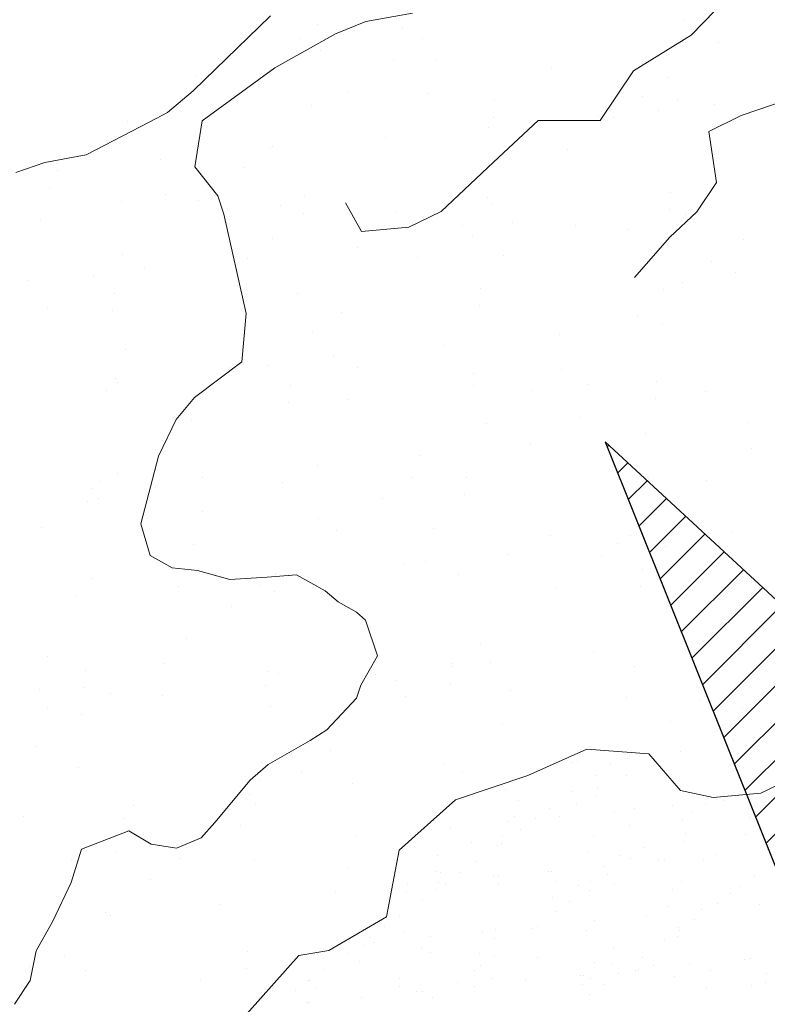
# Model space of a CAD drawing. Units: inches. Extents: x 1986 to 21484, y -1816 to 2016.
# Tile 62 of 85: x 3651.423 to 3655.81, y 1892.891 to 1898.672. Entities that reach past the tile are written whole.
import ezdxf

# ---------------------------------------------------------------- set-up
doc = ezdxf.new("R2010")
doc.units = ezdxf.units.IN
doc.layers.add('L-PLNT', color=84, linetype='Continuous', lineweight=13)
doc.layers.add('vfolhas', color=114, linetype='Continuous', lineweight=5)
doc.layers.add('vfolhas2', color=102, linetype='Continuous')

# ---------------------------------------------------------------- blocks, each defined once
blk = doc.blocks.new('arbusto_PB_verde_grande')
at = {"layer": 'vfolhas'}
h = blk.add_hatch(dxfattribs=at)
h.set_pattern_fill('ANSI31', color=256, scale=0.05, style=0)
h.set_pattern_definition([(45, (-2446.5133113, 50.986076), (-0.004419417382, 0.004419417382), [])])
h.paths.add_polyline_path([(-0.07279, 0.50669), (-0.18085, 0.65063), (-0.2334, 0.67253), (-0.20712, 0.53176), (-0.10785, 0.25007), (0.02625, -0.03934), (0.00028, 0.09048), (0.00816, 0.16241), (-0.04939, 0.29079)])
h.paths.add_polyline_path([(0.09902, 0.41929), (0.09372, 0.26573), (0.07906, 0.18814), (0.15506, 0.36901), (0.26606, 0.5505), (0.28356, 0.63504), (0.2485, 0.68819), (0.25145, 0.63504), (0.20178, 0.54426)])
h.paths.add_polyline_path([(0.12295, 0.24073), (0.047, 0.06233), (0.02625, -0.03934), (0.11122, 0.04358), (0.18428, 0.09364), (0.27478, 0.19376), (0.3215, 0.25323), (0.44129, 0.38467), (0.47634, 0.57866), (0.41789, 0.45347), (0.28939, 0.30954)])
h.paths.add_polyline_path([(0.58145, -0.03779), (0.70707, 0.01536), (0.78591, 0.04667), (0.74796, 0.06549), (0.62818, 0.08423), (0.52595, 0.09048), (0.39745, 0.04358), (0.02625, -0.03934), (0.25728, -0.03154), (0.43834, -0.0347)])
h.paths.add_polyline_path([(0.52022, -0.03647), (0.43834, -0.0347), (0.25728, -0.03154), (0.02625, -0.03934), (0.17964, -0.08515), (0.53768, -0.13167), (0.69541, -0.15357), (0.78591, -0.07852), (0.70413, -0.10042)])
h.paths.add_polyline_path([(0.27189, -0.21929), (0.14922, -0.14107), (0.02625, -0.03934), (0.15794, -0.31007), (0.29522, -0.42585), (0.41789, -0.49157), (0.56396, -0.56669), (0.5114, -0.48532), (0.39456, -0.34139)])
h.paths.add_polyline_path([(-0.05818, -0.47591), (-0.02312, -0.61984), (0.047, -0.80134), (0.08494, -0.59794), (0.07911, -0.4071), (0.03527, -0.25376), (0.02625, -0.03934), (-0.03773, -0.26001)])
h.paths.add_polyline_path([(-0.24218, 0.14054), (-0.11073, 0.06858), (0.02625, -0.03934), (-0.04235, 0.10871), (-0.21007, 0.23757), (-0.36485, 0.33145), (-0.47874, 0.40341), (-0.54303, 0.46288), (-0.49041, 0.33145), (-0.39408, 0.22192)])
at = {"layer": 'vfolhas2'}
for p, q in [((-0.54303, 0.46288), (-0.49041, 0.33145)), ((-0.47874, 0.40341), (-0.54303, 0.46288))]:
    blk.add_line(p, q, dxfattribs=at)
blk = doc.blocks.new('PLANT-SHRUB')
for p, q in [((2167.3863, 1874.3284), (2167.3863, 1874.3284)), ((2167.3494, 1874.2947), (2167.3494, 1874.2947)), ((2167.4592, 1874.2897), (2167.4592, 1874.2897)), ((2167.3538, 1874.1683), (2167.3538, 1874.1683)), ((2167.3823, 1874.1464), (2167.3823, 1874.1464)), ((2167.6597, 1874.1135), (2167.6597, 1874.1135)), ((2167.5754, 1874.0598), (2167.5754, 1874.0598)), ((2167.1002, 1873.9682), (2167.1002, 1873.9682)), ((2167.64, 1873.9488), (2167.64, 1873.9488)), ((2167.7513, 1873.937), (2167.7513, 1873.937)), ((2167.0085, 1873.8316), (2167.0085, 1873.8316)), ((2167.1125, 1873.8179), (2167.1125, 1873.8179)), ((2167.1125, 1873.8179), (2167.1125, 1873.8179)), ((2167.1794, 1873.8075), (2167.1794, 1873.8075)), ((2167.8017, 1873.8064), (2167.8017, 1873.8064)), ((2166.8467, 1873.7681), (2166.8467, 1873.7681)), ((2166.8467, 1873.7681), (2166.8467, 1873.7681)), ((2167.2749, 1873.7965), (2167.2749, 1873.7965)), ((2167.3697, 1873.7614), (2167.3697, 1873.7614)), ((2167.4374, 1873.7751), (2167.4374, 1873.7751)), ((2167.5464, 1873.7608), (2167.5464, 1873.7608)), ((2167.5774, 1873.7777), (2167.5774, 1873.7777)), ((2167.6504, 1873.7471), (2167.6504, 1873.7471)), ((2167.8809, 1873.7638), (2167.8809, 1873.7638)), ((2167.8928, 1873.7547), (2167.8928, 1873.7547)), ((2167.5406, 1873.744), (2167.5406, 1873.744)), ((2167.8129, 1873.7257), (2167.8129, 1873.7257)), ((2167.9803, 1873.7037), (2167.9803, 1873.7037)), ((2168.0843, 1873.69), (2168.0843, 1873.69)), ((2167.9692, 1873.6361), (2167.9692, 1873.6361)), ((2168.1883, 1873.6763), (2168.1883, 1873.6763)), ((2168.1883, 1873.6763), (2168.1883, 1873.6763)), ((2166.876, 1873.6143), (2166.876, 1873.6143)), ((2167.0876, 1873.5831), (2167.0876, 1873.5831)), ((2167.4983, 1873.6131), (2167.4983, 1873.6131)), ((2168.1206, 1873.612), (2168.1206, 1873.612)), ((2168.1782, 1873.6023), (2168.1782, 1873.6023)), ((2166.4493, 1873.5617), (2166.6467, 1873.5)), ((2166.7917, 1873.5606), (2166.7917, 1873.5606)), ((2167.1598, 1873.5541), (2167.1598, 1873.5541)), ((2167.3417, 1873.5617), (2167.3417, 1873.5617)), ((2167.414, 1873.5594), (2167.414, 1873.5594)), ((2167.6274, 1873.5637), (2167.6274, 1873.5637)), ((2167.8955, 1873.5686), (2167.8955, 1873.5686)), ((2168.0363, 1873.5583), (2168.0363, 1873.5583)), ((2168.1413, 1873.5686), (2168.1413, 1873.5686)), ((2168.1505, 1873.557), (2168.1505, 1873.557)), ((2166.6467, 1873.5), (2166.8689, 1873.3274)), ((2167.1678, 1873.4024), (2167.1678, 1873.4024)), ((2166.8341, 1873.383), (2166.8341, 1873.383)), ((2167.131, 1873.3687), (2167.131, 1873.3687)), ((2167.3286, 1873.3982), (2167.3286, 1873.3982)), ((2167.3572, 1873.3763), (2167.3572, 1873.3763)), ((2167.8684, 1873.3788), (2167.8684, 1873.3788)), ((2167.9424, 1873.3863), (2167.9424, 1873.3863)), ((2168.4081, 1873.3593), (2168.4081, 1873.3593)), ((2168.4081, 1873.3593), (2168.4081, 1873.3593)), ((2166.8689, 1873.3274), (2166.9799, 1873.1671)), ((2166.9282, 1873.3248), (2166.9282, 1873.3248)), ((2167.018, 1873.3071), (2167.018, 1873.3071)), ((2167.0907, 1873.3034), (2167.0907, 1873.3034)), ((2167.6403, 1873.306), (2167.6403, 1873.306)), ((2168.2626, 1873.3049), (2168.2626, 1873.3049)), ((2167.3621, 1873.2676), (2167.3621, 1873.2676)), ((2167.4661, 1873.254), (2167.4661, 1873.254)), ((2167.6286, 1873.2326), (2167.6286, 1873.2326)), ((2167.7686, 1873.227), (2167.7686, 1873.227)), ((2167.0751, 1873.1981), (2167.0751, 1873.1981)), ((2167.4977, 1873.2041), (2167.4977, 1873.2041)), ((2167.6148, 1873.1787), (2167.6148, 1873.1787)), ((2167.7317, 1873.1933), (2167.7317, 1873.1933)), ((2167.9, 1873.1968), (2167.9, 1873.1968)), ((2168.0041, 1873.1831), (2168.0041, 1873.1831)), ((2168.1379, 1873.172), (2168.1379, 1873.172)), ((2168.5431, 1873.2109), (2168.5431, 1873.2109)), ((2168.6491, 1873.1744), (2168.6491, 1873.1744)), ((2166.5531, 1873.1675), (2166.5531, 1873.1675)), ((2166.9799, 1873.1671), (2166.9676, 1872.8834)), ((2167.3369, 1873.1127), (2167.3369, 1873.1127)), ((2167.7977, 1873.1653), (2167.7977, 1873.1653)), ((2167.9592, 1873.1116), (2167.9592, 1873.1116)), ((2168.1665, 1873.1617), (2168.1665, 1873.1617)), ((2168.438, 1873.126), (2168.438, 1873.126)), ((2168.542, 1873.1123), (2168.542, 1873.1123)), ((2168.5815, 1873.1105), (2168.5815, 1873.1105)), ((2166.3845, 1873.0602), (2166.3845, 1873.0602)), ((2167.2526, 1873.059), (2167.2526, 1873.059)), ((2167.6292, 1873.0579), (2167.6292, 1873.0579)), ((2167.875, 1873.0579), (2167.875, 1873.0579)), ((2168.4973, 1873.0568), (2168.4973, 1873.0568)), ((2168.7044, 1873.0909), (2168.7044, 1873.0909)), ((2168.8738, 1873.0556), (2168.8738, 1873.0556)), ((2166.8215, 1872.998), (2166.8215, 1872.998)), ((2167.5328, 1873.011), (2167.5328, 1873.011)), ((2168.3325, 1873.0179), (2168.3325, 1873.0179)), ((2168.3693, 1873.0516), (2168.3693, 1873.0516)), ((2167.3446, 1872.9913), (2167.3446, 1872.9913)), ((2167.8558, 1872.9937), (2167.8558, 1872.9937)), ((2167.8677, 1872.9846), (2167.8677, 1872.9846)), ((2168.3955, 1872.9743), (2168.3955, 1872.9743)), ((2168.8901, 1872.9895), (2168.8901, 1872.9895)), ((2168.9186, 1872.9676), (2168.9186, 1872.9676)), ((2166.9676, 1872.8834), (2167.2144, 1872.6121)), ((2167.15, 1872.8855), (2167.15, 1872.8855)), ((2166.536, 1872.859), (2166.536, 1872.859)), ((2166.744, 1872.8316), (2166.744, 1872.8316)), ((2167.359, 1872.8517), (2167.359, 1872.8517)), ((2168.1336, 1872.8356), (2168.1336, 1872.8356)), ((2168.6992, 1872.8533), (2168.6992, 1872.8533)), ((2168.9332, 1872.8425), (2168.9332, 1872.8425)), ((2168.97, 1872.8762), (2168.97, 1872.8762)), ((2167.0625, 1872.8131), (2167.0625, 1872.8131)), ((2167.0689, 1872.7888), (2167.0689, 1872.7888)), ((2167.0763, 1872.818), (2167.0763, 1872.818)), ((2167.1779, 1872.7745), (2167.1779, 1872.7745)), ((2167.3221, 1872.818), (2167.3221, 1872.818)), ((2167.4789, 1872.8056), (2167.4789, 1872.8056)), ((2167.6022, 1872.7936), (2167.6022, 1872.7936)), ((2168.1012, 1872.8044), (2168.1012, 1872.8044)), ((2168.1253, 1872.7869), (2168.1253, 1872.7869)), ((2168.6365, 1872.7894), (2168.6365, 1872.7894)), ((2168.7235, 1872.8033), (2168.7235, 1872.8033)), ((2169.1762, 1872.7699), (2169.1762, 1872.7699)), ((2167.2819, 1872.7608), (2167.2819, 1872.7608)), ((2167.4444, 1872.7394), (2167.4444, 1872.7394)), ((2167.6118, 1872.7174), (2167.6118, 1872.7174)), ((2167.7158, 1872.7037), (2167.7158, 1872.7037)), ((2167.8198, 1872.69), (2167.8198, 1872.69)), ((2167.8198, 1872.69), (2167.8198, 1872.69)), ((2167.9597, 1872.6763), (2167.9597, 1872.6763)), ((2167.9823, 1872.6686), (2167.9823, 1872.6686)), ((2168.7343, 1872.6602), (2168.7343, 1872.6602)), ((2166.2811, 1872.6232), (2166.2811, 1872.6232)), ((2167.2144, 1872.6121), (2167.5723, 1872.4888)), ((2167.2144, 1872.6121), (2167.2144, 1872.6121)), ((2167.3034, 1872.6281), (2167.3034, 1872.6281)), ((2167.332, 1872.6062), (2167.332, 1872.6062)), ((2167.7978, 1872.6112), (2167.7978, 1872.6112)), ((2167.8432, 1872.6087), (2167.8432, 1872.6087)), ((2167.9229, 1872.6426), (2167.9229, 1872.6426)), ((2168.1447, 1872.6472), (2168.1447, 1872.6472)), ((2168.2537, 1872.6329), (2168.2537, 1872.6329)), ((2168.3577, 1872.6192), (2168.3577, 1872.6192)), ((2168.4201, 1872.61), (2168.4201, 1872.61)), ((2168.5202, 1872.5978), (2168.5202, 1872.5978)), ((2169.0425, 1872.6089), (2169.0425, 1872.6089)), ((2166.837, 1872.5533), (2166.837, 1872.5533)), ((2167.7136, 1872.5575), (2167.7136, 1872.5575)), ((2168.0817, 1872.551), (2168.0817, 1872.551)), ((2168.3359, 1872.5564), (2168.3359, 1872.5564)), ((2168.3515, 1872.5347), (2168.3515, 1872.5347)), ((2168.3829, 1872.5893), (2168.3829, 1872.5893)), ((2168.3829, 1872.5893), (2168.3829, 1872.5893)), ((2168.6876, 1872.5757), (2168.6876, 1872.5757)), ((2168.7916, 1872.562), (2168.7916, 1872.562)), ((2168.8956, 1872.5484), (2168.8956, 1872.5484)), ((2168.8956, 1872.5484), (2168.8956, 1872.5484)), ((2168.906, 1872.5826), (2168.906, 1872.5826)), ((2168.9582, 1872.5552), (2168.9582, 1872.5552)), ((2169.3263, 1872.5487), (2169.3263, 1872.5487)), ((2169.4172, 1872.585), (2169.4172, 1872.585)), ((2169.4291, 1872.5759), (2169.4291, 1872.5759)), ((2167.5723, 1872.4888), (2167.9796, 1872.3039)), ((2168.4239, 1872.2915), (2168.7447, 1872.5258)), ((2168.5604, 1872.5009), (2168.5604, 1872.5009)), ((2168.7447, 1872.5258), (2169.1273, 1872.4395)), ((2169.0581, 1872.527), (2169.0581, 1872.527)), ((2169.2206, 1872.5056), (2169.2206, 1872.5056)), ((2169.3295, 1872.4912), (2169.3295, 1872.4912)), ((2169.335, 1872.4848), (2169.335, 1872.4848)), ((2169.4335, 1872.4775), (2169.4335, 1872.4775)), ((2166.6785, 1872.4534), (2166.6785, 1872.4534)), ((2167.724, 1872.4603), (2167.724, 1872.4603)), ((2168.2778, 1872.4672), (2168.2778, 1872.4672)), ((2168.5236, 1872.4672), (2168.5236, 1872.4672)), ((2169.1273, 1872.4395), (2169.2754, 1872.3408)), ((2168.1127, 1872.4019), (2168.1127, 1872.4019)), ((2169.2754, 1872.3408), (2169.8431, 1872.3902)), ((2167.9796, 1872.3039), (2168.4239, 1872.2915)), ((2165.7168, 1872.2668), (2165.7168, 1872.2668)), ((2166.7963, 1872.2279), (2166.7963, 1872.2279)), ((2167.8425, 1872.2145), (2167.8425, 1872.2145)), ((2168.8649, 1872.2194), (2168.8649, 1872.2194)), ((2166.2303, 1872.1667), (2166.2303, 1872.1667)), ((2166.3308, 1872.1348), (2166.3308, 1872.1348)), ((2167.4749, 1872.1645), (2167.4749, 1872.1645)), ((2168.7195, 1872.1622), (2168.7195, 1872.1622)), ((2169.5529, 1872.1839), (2169.5529, 1872.1839)), ((2167.88, 1872.1027), (2167.88, 1872.1027)), ((2169.4793, 1872.1164), (2169.4793, 1872.1164)), ((2166.0617, 1872.0593), (2166.0617, 1872.0593)), ((2166.2572, 1872.0673), (2166.2572, 1872.0673)), ((2167.3064, 1872.0571), (2167.3064, 1872.0571)), ((2168.551, 1872.0548), (2168.551, 1872.0548)), ((2169.7956, 1872.0526), (2169.7956, 1872.0526)), ((2165.2997, 1871.987), (2165.2997, 1871.987)), ((2165.6246, 1871.9442), (2165.6246, 1871.9442)), ((2165.2097, 1871.8665), (2165.2097, 1871.8665)), ((2166.1675, 1871.8727), (2166.1675, 1871.8727)), ((2166.2559, 1871.8531), (2166.2559, 1871.8531)), ((2166.3755, 1871.8453), (2166.3755, 1871.8453)), ((2167.2783, 1871.858), (2167.2783, 1871.858)), ((2166.7004, 1871.8025), (2166.7004, 1871.8025)), ((2167.5323, 1871.784), (2167.5323, 1871.784)), ((2168.3577, 1871.8192), (2168.3577, 1871.8192)), ((2169.4039, 1871.8058), (2169.4039, 1871.8058)), ((2167.2433, 1871.7311), (2167.2433, 1871.7311)), ((2169.0815, 1871.7519), (2169.0815, 1871.7519)), ((2165.8594, 1871.7028), (2165.8594, 1871.7028)), ((2167.4513, 1871.7037), (2167.4513, 1871.7037)), ((2167.4586, 1871.7165), (2167.4586, 1871.7165)), ((2167.7762, 1871.6609), (2167.7762, 1871.6609)), ((2165.2696, 1871.5547), (2165.2696, 1871.5547)), ((2166.5142, 1871.5524), (2166.5142, 1871.5524)), ((2167.7589, 1871.5502), (2167.7589, 1871.5502)), ((2168.3191, 1871.5894), (2168.3191, 1871.5894)), ((2168.5271, 1871.5621), (2168.5271, 1871.5621)), ((2165.6917, 1871.4967), (2165.6917, 1871.4967)), ((2168.8521, 1871.5193), (2168.8521, 1871.5193)), ((2169.0035, 1871.5479), (2169.0035, 1871.5479)), ((2170.2481, 1871.5457), (2170.2481, 1871.5457)), ((2166.7711, 1871.4578), (2166.7711, 1871.4578)), ((2167.8173, 1871.4444), (2167.8173, 1871.4444)), ((2167.9246, 1871.4318), (2167.995, 1871.4697)), ((2167.995, 1871.4697), (2168.2495, 1871.4859)), ((2168.2495, 1871.4859), (2168.3632, 1871.4643)), ((2168.3632, 1871.4643), (2168.6394, 1871.3994)), ((2168.8397, 1871.4493), (2168.8397, 1871.4493)), ((2169.1015, 1871.4329), (2169.2206, 1871.4437)), ((2169.2206, 1871.4437), (2169.3668, 1871.3896)), ((2169.3949, 1871.4478), (2169.3949, 1871.4478)), ((2165.5117, 1871.3842), (2165.5117, 1871.3842)), ((2167.7351, 1871.3723), (2167.9246, 1871.4318)), ((2168.6394, 1871.3994), (2168.7801, 1871.394)), ((2168.7338, 1871.4333), (2168.7338, 1871.4333)), ((2168.7801, 1871.394), (2169.1015, 1871.4329)), ((2169.3668, 1871.3896), (2169.4589, 1871.2705)), ((2169.603, 1871.4204), (2169.603, 1871.4204)), ((2169.9192, 1871.4104), (2169.9192, 1871.4104)), ((2169.9279, 1871.3776), (2169.9279, 1871.3776)), ((2170.2829, 1871.4011), (2170.2829, 1871.4011)), ((2170.5256, 1871.3679), (2170.6881, 1871.4058)), ((2167.0608, 1871.352), (2167.0608, 1871.352)), ((2167.643, 1871.1721), (2167.7351, 1871.3723)), ((2168.6601, 1871.3658), (2168.6601, 1871.3658)), ((2170.3794, 1871.2651), (2170.5256, 1871.3679)), ((2165.438, 1871.3167), (2165.438, 1871.3167)), ((2169.4589, 1871.2705), (2169.5022, 1871.1244)), ((2170.1899, 1871.2056), (2170.3794, 1871.2651)), ((2170.4708, 1871.3062), (2170.4708, 1871.3062)), ((2169.9571, 1871.1136), (2170.1899, 1871.2056)), ((2164.6629, 1871.1682), (2164.6629, 1871.1682)), ((2165.9075, 1871.1659), (2165.9075, 1871.1659)), ((2167.1521, 1871.1636), (2167.1521, 1871.1636)), ((2167.6484, 1871.1018), (2167.643, 1871.1721)), ((2168.3968, 1871.1614), (2168.3968, 1871.1614)), ((2169.6414, 1871.1591), (2169.6414, 1871.1591)), ((2165.1845, 1871.0964), (2165.1845, 1871.0964)), ((2167.2531, 1871.0879), (2167.2531, 1871.0879)), ((2167.6863, 1870.9827), (2167.6484, 1871.1018)), ((2169.5022, 1871.1244), (2169.7784, 1871.0108)), ((2169.7784, 1871.0108), (2169.9571, 1871.1136)), ((2164.4943, 1871.0608), (2164.4943, 1871.0608)), ((2165.739, 1871.0585), (2165.739, 1871.0585)), ((2166.2307, 1871.083), (2166.2307, 1871.083)), ((2166.7131, 1871.0334), (2166.7131, 1871.0334)), ((2166.9836, 1871.0563), (2166.9836, 1871.0563)), ((2168.2282, 1871.054), (2168.2282, 1871.054)), ((2168.3326, 1871.0491), (2168.3326, 1871.0491)), ((2169.3787, 1871.0357), (2169.3787, 1871.0357)), ((2169.4729, 1871.0517), (2169.4729, 1871.0517)), ((2169.9352, 1871.0825), (2169.9352, 1871.0825)), ((2164.7231, 1871.0281), (2164.7231, 1871.0281)), ((2164.9312, 1871.0007), (2164.9312, 1871.0007)), ((2167.6972, 1870.8854), (2167.6863, 1870.9827)), ((2168.2623, 1871.0012), (2168.2623, 1871.0012)), ((2169.8616, 1871.015), (2169.8616, 1871.015)), ((2165.0402, 1870.9522), (2165.0402, 1870.9522)), ((2165.2561, 1870.9579), (2165.2561, 1870.9579)), ((2166.6394, 1870.9659), (2166.6394, 1870.9659)), ((2165.799, 1870.8864), (2165.799, 1870.8864)), ((2166.007, 1870.859), (2166.007, 1870.859)), ((2167.7567, 1870.7014), (2167.6972, 1870.8854)), ((2166.3319, 1870.8163), (2166.3319, 1870.8163)), ((2164.3818, 1870.708), (2164.5846, 1870.7548)), ((2164.5846, 1870.7548), (2164.8029, 1870.7548)), ((2164.8029, 1870.7548), (2165.1149, 1870.7859)), ((2165.1149, 1870.7859), (2165.1149, 1870.7859)), ((2166.8748, 1870.7448), (2166.8748, 1870.7448)), ((2163.5552, 1870.7236), (2164.0075, 1870.521)), ((2164.2103, 1870.4587), (2164.3818, 1870.708)), ((2164.6441, 1870.7217), (2164.6441, 1870.7217)), ((2165.6665, 1870.7266), (2165.6665, 1870.7266)), ((2166.746, 1870.6877), (2166.746, 1870.6877)), ((2167.0828, 1870.7174), (2167.0828, 1870.7174)), ((2167.8921, 1870.5932), (2167.7567, 1870.7014)), ((2167.9146, 1870.6826), (2167.9146, 1870.6826)), ((2164.6925, 1870.6335), (2164.6925, 1870.6335)), ((2167.4077, 1870.6746), (2167.4077, 1870.6746)), ((2167.7921, 1870.6743), (2167.7921, 1870.6743)), ((2168.8145, 1870.6792), (2168.8145, 1870.6792)), ((2169.4637, 1870.6505), (2169.4637, 1870.6505)), ((2169.894, 1870.6403), (2169.894, 1870.6403)), ((2166.2416, 1870.6014), (2166.2416, 1870.6014)), ((2167.8409, 1870.6151), (2167.8409, 1870.6151)), ((2168.06, 1870.4525), (2167.8921, 1870.5932)), ((2167.9506, 1870.6031), (2167.9506, 1870.6031)), ((2168.1586, 1870.5758), (2168.1586, 1870.5758)), ((2164.0075, 1870.521), (2164.2103, 1870.4587)), ((2164.6188, 1870.566), (2164.6188, 1870.566)), ((2164.9468, 1870.5539), (2164.9468, 1870.5539)), ((2166.1915, 1870.5516), (2166.1915, 1870.5516)), ((2167.4361, 1870.5494), (2167.4361, 1870.5494)), ((2168.4836, 1870.533), (2168.4836, 1870.533)), ((2168.6807, 1870.5471), (2168.6807, 1870.5471)), ((2168.1629, 1870.2848), (2168.06, 1870.4525)), ((2169.0264, 1870.4615), (2169.0264, 1870.4615)), ((2169.2345, 1870.4341), (2169.2345, 1870.4341)), ((2164.0799, 1870.3652), (2164.0799, 1870.3652)), ((2169.5594, 1870.3913), (2169.5594, 1870.3913)), ((2165.1593, 1870.3263), (2165.1593, 1870.3263)), ((2165.8939, 1870.2828), (2165.8939, 1870.2828)), ((2166.2055, 1870.313), (2166.2055, 1870.313)), ((2167.2279, 1870.3179), (2167.2279, 1870.3179)), ((2168.2603, 1870.1712), (2168.1629, 1870.2848)), ((2168.3074, 1870.279), (2168.3074, 1870.279)), ((2169.116, 1870.3318), (2169.116, 1870.3318)), ((2167.4431, 1870.2506), (2167.4431, 1870.2506)), ((2169.0424, 1870.2643), (2169.0424, 1870.2643)), ((2169.3536, 1870.2656), (2169.3536, 1870.2656)), ((2164.221, 1870.2015), (2164.221, 1870.2015)), ((2164.3401, 1870.1673), (2164.3401, 1870.1673)), ((2165.5847, 1870.1651), (2165.5847, 1870.1651)), ((2165.8203, 1870.2153), (2165.8203, 1870.2153)), ((2166.8293, 1870.1628), (2166.8293, 1870.1628)), ((2168.3036, 1870.0305), (2168.2603, 1870.1712)), ((2163.8118, 1870.1132), (2163.8118, 1870.1132)), ((2168.074, 1870.1606), (2168.074, 1870.1606)), ((2169.3186, 1870.1583), (2169.3186, 1870.1583)), ((2164.1715, 1870.06), (2164.1715, 1870.06)), ((2165.4162, 1870.0577), (2165.4162, 1870.0577)), ((2166.6608, 1870.0554), (2166.6608, 1870.0554)), ((2167.9054, 1870.0532), (2167.9054, 1870.0532)), ((2169.1501, 1870.0509), (2169.1501, 1870.0509)), ((2164.3546, 1870.0418), (2164.3546, 1870.0418)), ((2164.5627, 1870.0144), (2164.5627, 1870.0144)), ((2168.217, 1869.8573), (2168.3036, 1870.0305)), ((2163.8984, 1869.9755), (2163.5552, 1869.96)), ((2164.2883, 1869.8976), (2163.8984, 1869.9755)), ((2164.6314, 1869.9755), (2164.2883, 1869.8976)), ((2164.6189, 1869.9516), (2164.6189, 1869.9516)), ((2164.8965, 1869.7262), (2164.6314, 1869.9755)), ((2164.8876, 1869.9716), (2164.8876, 1869.9716)), ((2165.6413, 1869.9565), (2165.6413, 1869.9565)), ((2167.0954, 1869.932), (2167.0954, 1869.932)), ((2163.8733, 1869.8829), (2163.8733, 1869.8829)), ((2165.4305, 1869.9001), (2165.4305, 1869.9001)), ((2165.6385, 1869.8727), (2165.6385, 1869.8727)), ((2166.7208, 1869.9176), (2166.7208, 1869.9176)), ((2167.767, 1869.9042), (2167.767, 1869.9042)), ((2168.6446, 1869.8998), (2168.6446, 1869.8998)), ((2168.7893, 1869.9091), (2168.7893, 1869.9091)), ((2165.4225, 1869.8507), (2165.4225, 1869.8507)), ((2165.9634, 1869.83), (2165.9634, 1869.83)), ((2167.0217, 1869.8645), (2167.0217, 1869.8645)), ((2167.8695, 1869.6393), (2168.217, 1869.8573)), ((2166.5063, 1869.7585), (2166.5063, 1869.7585)), ((2165.2552, 1869.7262), (2164.8965, 1869.7262)), ((2165.2552, 1869.7262), (2165.2552, 1869.7262)), ((2165.6763, 1869.7262), (2165.2552, 1869.7262)), ((2165.8791, 1869.6639), (2165.6763, 1869.7262)), ((2166.7143, 1869.7311), (2166.7143, 1869.7311)), ((2166.0974, 1869.4924), (2165.8791, 1869.6639)), ((2167.0393, 1869.6883), (2167.0393, 1869.6883)), ((2167.5821, 1869.6169), (2167.5821, 1869.6169)), ((2167.6475, 1869.5527), (2167.8695, 1869.6393)), ((2167.7902, 1869.5895), (2167.7902, 1869.5895)), ((2164.624, 1869.5531), (2164.624, 1869.5531)), ((2165.0748, 1869.5321), (2165.0748, 1869.5321)), ((2165.1342, 1869.5562), (2165.1342, 1869.5562)), ((2165.8687, 1869.5508), (2165.8687, 1869.5508)), ((2166.1803, 1869.5429), (2166.1803, 1869.5429)), ((2166.9219, 1869.3796), (2167.1331, 1869.569)), ((2167.1133, 1869.5485), (2167.1133, 1869.5485)), ((2167.1331, 1869.569), (2167.4797, 1869.5311)), ((2167.2027, 1869.5478), (2167.2027, 1869.5478)), ((2167.4797, 1869.5311), (2167.6475, 1869.5527)), ((2168.1151, 1869.5467), (2168.1151, 1869.5467)), ((2168.2969, 1869.5812), (2168.2969, 1869.5812)), ((2168.3579, 1869.5463), (2168.3579, 1869.5463)), ((2166.0506, 1869.3054), (2166.0974, 1869.4924)), ((2166.6239, 1869.5), (2166.6239, 1869.5)), ((2168.2232, 1869.5137), (2168.2232, 1869.5137)), ((2168.2822, 1869.5089), (2168.2822, 1869.5089)), ((2168.6579, 1869.4752), (2168.6579, 1869.4752)), ((2165.0011, 1869.4646), (2165.0011, 1869.4646)), ((2166.6174, 1868.8651), (2166.9219, 1869.3796)), ((2165.6161, 1869.1864), (2165.6161, 1869.1864)), ((2166.2762, 1869.1813), (2166.2762, 1869.1813)), ((2165.2619, 1869.1643), (2165.2619, 1869.1643)), ((2166.5066, 1869.162), (2166.5066, 1869.162)), ((2166.6956, 1869.1475), (2166.6956, 1869.1475)), ((2167.7418, 1869.1341), (2167.7418, 1869.1341)), ((2167.7512, 1869.1597), (2167.7512, 1869.1597)), ((2167.8254, 1869.1492), (2167.8254, 1869.1492)), ((2166.2026, 1869.1138), (2166.2026, 1869.1138)), ((2165.0934, 1869.0569), (2165.0934, 1869.0569)), ((2166.338, 1869.0546), (2166.338, 1869.0546)), ((2167.5827, 1869.0524), (2167.5827, 1869.0524)), ((2165.062, 1868.9138), (2165.062, 1868.9138)), ((2165.27, 1868.8864), (2165.27, 1868.8864)), ((2165.5949, 1868.8437), (2165.5949, 1868.8437)), ((2166.5687, 1868.7623), (2166.6174, 1868.8651)), ((2165.109, 1868.7861), (2165.109, 1868.7861)), ((2167.1776, 1868.7777), (2167.1776, 1868.7777)), ((2167.4777, 1868.8306), (2167.4777, 1868.8306)), ((2165.0038, 1868.7623), (2165.2367, 1868.6108)), ((2165.8048, 1868.7493), (2165.8048, 1868.7493)), ((2166.1378, 1868.7722), (2166.1378, 1868.7722)), ((2166.1552, 1868.7728), (2166.1552, 1868.7728)), ((2166.3458, 1868.7448), (2166.3458, 1868.7448)), ((2166.5525, 1868.5459), (2166.5687, 1868.7623)), ((2167.404, 1868.7631), (2167.404, 1868.7631)), ((2166.6708, 1868.702), (2166.6708, 1868.702)), ((2165.2367, 1868.6108), (2165.4154, 1868.5405)), ((2167.2136, 1868.6306), (2167.2136, 1868.6306)), ((2167.4217, 1868.6032), (2167.4217, 1868.6032)), ((2165.5459, 1868.55), (2165.5459, 1868.55)), ((2166.3359, 1868.3781), (2166.5525, 1868.5459)), ((2166.7905, 1868.5477), (2166.7905, 1868.5477)), ((2167.7466, 1868.5604), (2167.7466, 1868.5604)), ((2165.4154, 1868.5405), (2165.8106, 1868.4431)), ((2165.457, 1868.4307), (2165.457, 1868.4307)), ((2165.8106, 1868.4431), (2166.3359, 1868.3781)), ((2165.591, 1868.4163), (2165.591, 1868.4163)), ((2166.6704, 1868.3774), (2166.6704, 1868.3774)), ((2167.0062, 1868.3985), (2167.0062, 1868.3985)), ((2167.7166, 1868.364), (2167.7166, 1868.364)), ((2166.2531, 1868.2145), (2165.6213, 1868.2041)), ((2166.4499, 1868.2041), (2166.2531, 1868.2145)), ((2166.5638, 1868.1731), (2166.4499, 1868.2041)), ((2166.1838, 1868.1612), (2166.1838, 1868.1612)), ((2166.5638, 1868.1731), (2166.5638, 1868.1731)), ((2166.9677, 1868.0592), (2166.5638, 1868.1731)), ((2167.4284, 1868.1589), (2167.4284, 1868.1589)), ((2166.6585, 1868.0799), (2166.6585, 1868.0799)), ((2166.9677, 1868.0592), (2166.9677, 1868.0592)), ((2167.1749, 1867.9247), (2166.9677, 1868.0592)), ((2167.2599, 1868.0516), (2167.2599, 1868.0516)), ((2167.1524, 1868.0076), (2167.1524, 1868.0076)), ((2167.3406, 1867.8522), (2167.1749, 1867.9247))]:
    blk.add_line(p, q)

msp = doc.modelspace()

# ---------------------------------------------------------------- block references
at = {"layer": 'L-PLNT', "rotation": 223.1883365522388}
msp.add_blockref('PLANT-SHRUB', (3953.27, 4742.9646), dxfattribs=at)
at = {"layer": 'L-PLNT', "xscale": 24.60366729364114, "yscale": 24.60366729364114, "zscale": 24.60366729364114}
msp.add_blockref('arbusto_PB_verde_grande', (3668.2184, 1884.8051), dxfattribs=at)

doc.saveas('drawing.dxf')
